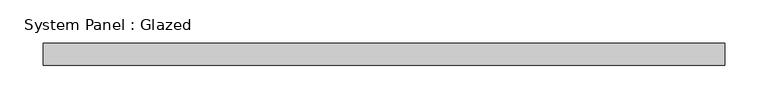
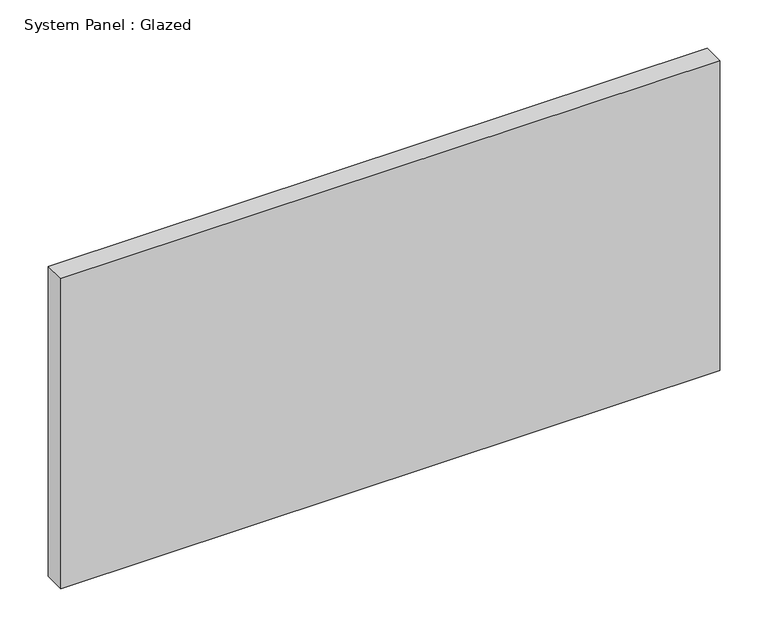
"""IFC4 building model written with IfcOpenShell, lengths in millimetres: plate geometry, System Panel : Glazed."""

from ifc_helpers import new_model, si_unit, origin, origin_with_axes, place, context, project, spatial, polyline, outline, extrude, source, transform, mapped, element, save


def system_panel_glazed_23dedc8c(model_context):
    return source(origin(), model_context, "Body", "SweptSolid", [
        extrude(outline(polyline([(393.7, 19.05), (-393.7, 19.05), (-393.7, 44.45), (393.7, 44.45), (393.7, 19.05)])), origin_with_axes(), (0.0, 0.0, 1.0), 391.9090709),
    ])


if __name__ == "__main__":
    model = new_model("IFC4")
    model_context = context("Model", 3, world=origin())
    ifc_project = project(units=[si_unit("LENGTHUNIT", "METRE", prefix="MILLI")], contexts=[model_context])
    site = spatial("IfcSite", under=ifc_project)
    building = spatial("IfcBuilding", under=site)
    placement = place(None, origin())
    system_panel_glazed_shape = system_panel_glazed_23dedc8c(model_context)
    element("IfcPlate", 1, ObjectType="System Panel : Glazed", at=placement, inside=building, context=model_context, shape_type="MappedRepresentation", body=[
        mapped(system_panel_glazed_shape, transform((0.0, 0.0, 0.0), x_axis=(1.0, 0.0, 0.0), y_axis=(0.0, 1.0, 0.0), z_axis=(0.0, 0.0, 1.0))),
    ])
    save(model, "model.ifc")

# Revit data of these elements
# Type "System Panel : Glazed"
#   Construction Type Id = "GSP4R"
#   Analytic Construction = "1/8 in Pilkington single glazing"
#   Visual Light Transmittance = 0.9
#   Solar Heat Gain Coefficient = 0.86
#   Heat Transfer Coefficient (U) = 1.18115 BTU/(h·ft²·°F)
# Element 1 (IfcPlate, "System Panel : Glazed")
#   Materials on its faces: "Glass"
# Materials
#   "Glass": class "Glass", colour RGB 0 128 192, transparency 0.75, Description = "Soda Lime Glass", Cost = 0
